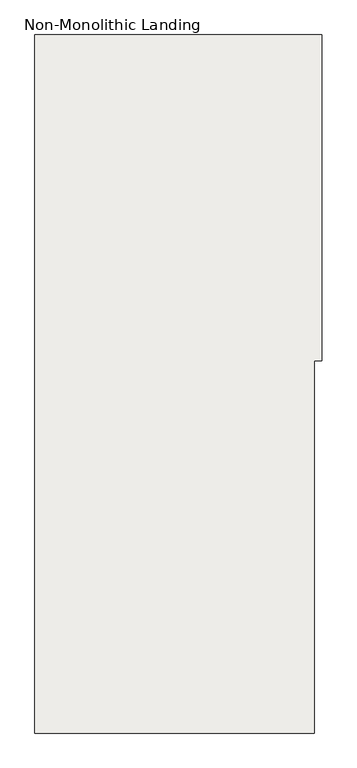
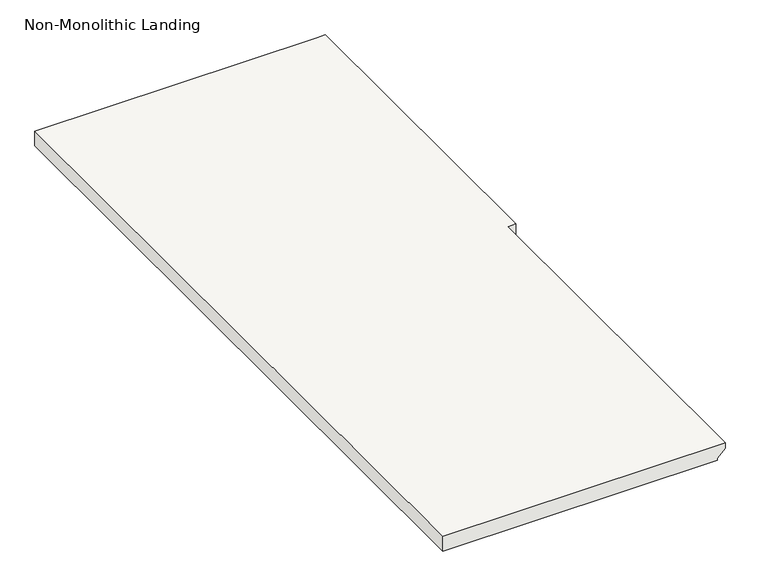
"""IFC4 building model written with IfcOpenShell, lengths in millimetres: slab geometry, Non-Monolithic Landing."""

from ifc_helpers import new_model, si_unit, origin, place, context, project, spatial, faceted_brep, source, transform, mapped, element, save


def non_monolithic_landing_bbfcd8c5(model_context):
    return source(origin(), model_context, "Body", "Brep", [
        faceted_brep([(-13376.4750862, 7319.8620171, 1354.6666667), (-13351.0750862, 7319.8620171, 1354.6666667), (-13351.0750862, 8386.6620171, 1354.6666667), (-13376.4750862, 8386.6620171, 1354.6666667), (-14290.8750862, 8386.6620171, 1354.6666667), (-14290.8750862, 6100.6620171, 1354.6666667), (-13376.4750862, 6100.6620171, 1354.6666667), (-13401.8750862, 7015.0620171, 1303.8666667), (-13401.8750862, 6100.6620171, 1303.8666667), (-14290.8750862, 6100.6620171, 1303.8666667), (-14290.8750862, 8386.6620171, 1303.8666667), (-13376.4750862, 8386.6620171, 1303.8666667), (-13351.0750862, 8386.6620171, 1303.8666667), (-13351.0750862, 7319.8620171, 1303.8666667), (-13376.4750862, 7319.8620171, 1303.8666667), (-13376.4750862, 7015.0620171, 1303.8666667), (-13401.8750862, 6100.6620171, 1310.2166667), (-13376.4750862, 6100.6620171, 1335.6166667), (-13376.4750862, 7015.0620171, 1335.6166667), (-13401.8750862, 7015.0620171, 1310.2166667)], [[[0, 1, 2, 3, 4, 5, 6]], [[7, 8, 9, 10, 11, 12, 13, 14, 15]], [[6, 5, 9, 8, 16, 17]], [[0, 6, 17, 18, 15, 14]], [[3, 2, 12, 11]], [[2, 1, 13, 12]], [[4, 3, 11, 10]], [[5, 4, 10, 9]], [[17, 16, 19, 18]], [[8, 7, 19, 16]], [[7, 15, 18, 19]], [[1, 0, 14, 13]]]),
    ])


if __name__ == "__main__":
    model = new_model("IFC4")
    model_context = context("Model", 3, world=origin())
    ifc_project = project(units=[si_unit("LENGTHUNIT", "METRE", prefix="MILLI")], contexts=[model_context])
    site = spatial("IfcSite", under=ifc_project)
    building = spatial("IfcBuilding", under=site)
    placement = place(None, origin())
    non_monolithic_landing_shape = non_monolithic_landing_bbfcd8c5(model_context)
    element("IfcSlab", 1, ObjectType="Non-Monolithic Landing", at=placement, inside=building, context=model_context, shape_type="MappedRepresentation", body=[
        mapped(non_monolithic_landing_shape, transform((0.0, 0.0, 0.0), x_axis=(1.0, 0.0, 0.0), y_axis=(0.0, 1.0, 0.0), z_axis=(0.0, 0.0, 1.0))),
    ])
    save(model, "model.ifc")
